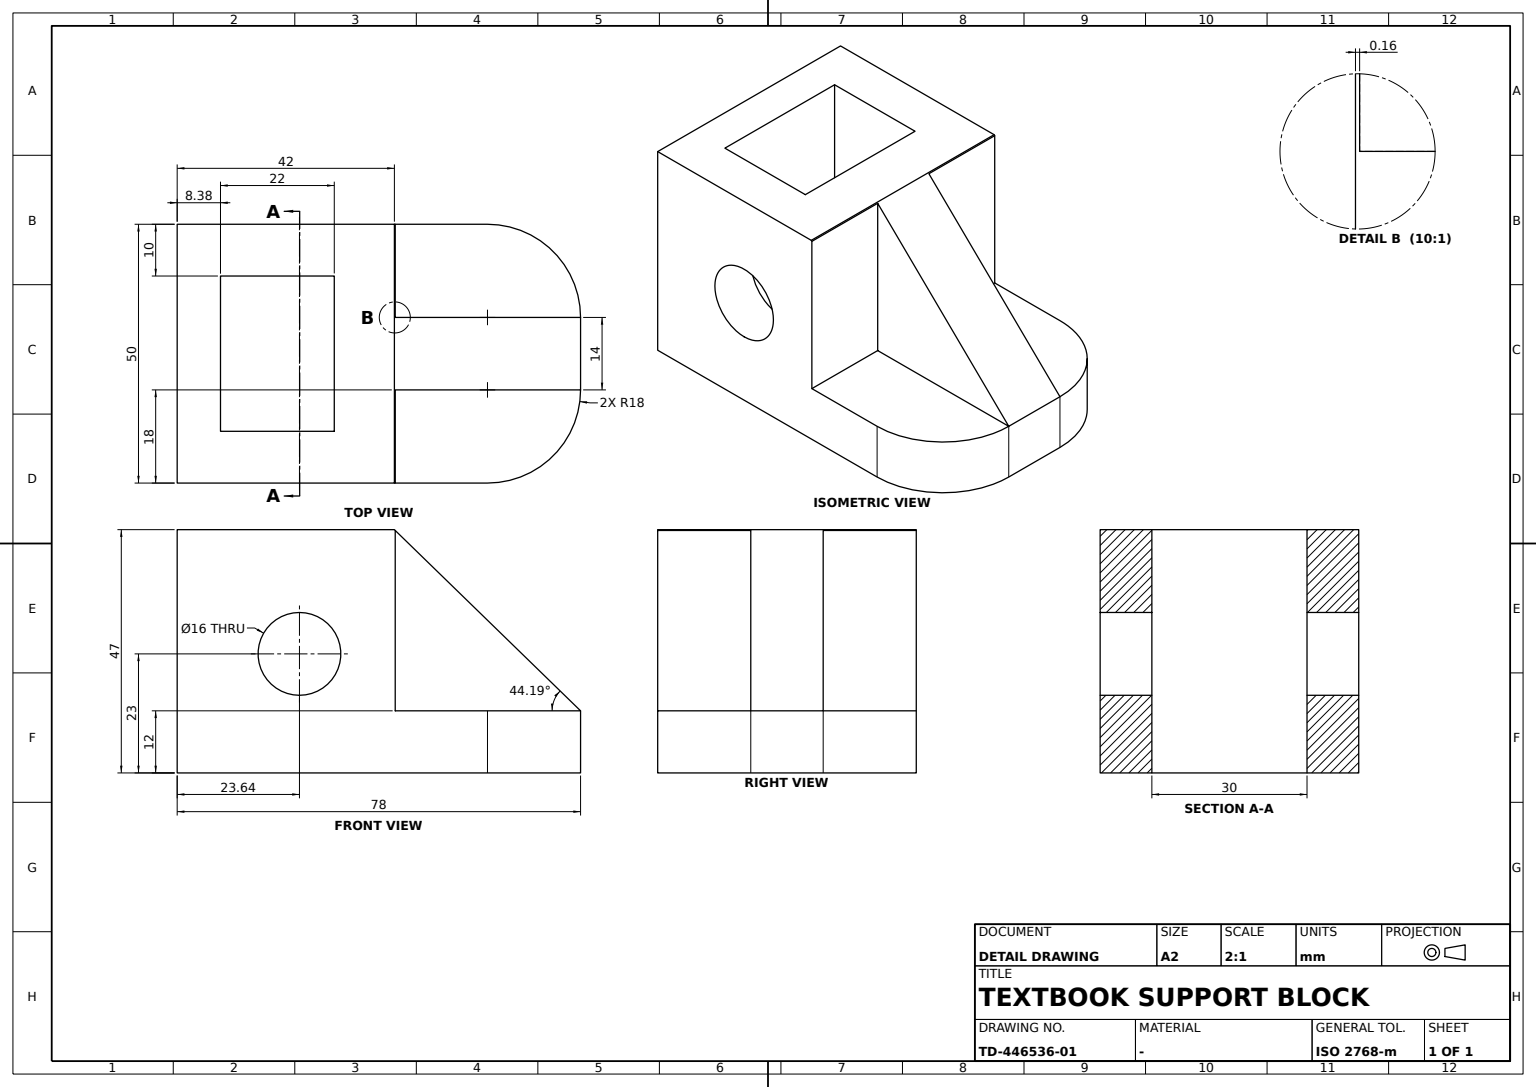
CATIA V5 part; units mm, degrees
sketch "Sketch1" plane through (0, 0, 0) normal (1, 0, 0) x (0, 1, 0)
  line L0 (0, 0) -> (0, 47)
  line L1 (0, 47) -> (78, 47)
  line L2 (78, 47) -> (78, 0)
  point P0 (78, 0)
  line L3 (78, 0) -> (0, 0)
  dimension "length L0" = 47
  dimension "length L3" = 78
  dimension "length L2" = 47
  dimension "length L1" = 78
  constraint vertical L0 y-axis
  constraint vertical L2 y-axis
  constraint horizontal L1 x-axis
  constraint horizontal L3 x-axis
  constraint coincidence P0 x-axis
extrude "Pad1" add sketch "Sketch1" along normal mid plane 50
sketch "Sketch2" plane through (25, 0, 0) normal (1, 0, 0) x (0, 1, 0)
  point P0 (42, 47)
  line L0 (42, 47) -> (78, 12)
  point P1 (78, 12)
  line L1 (78, 12) -> (78, 47)
  line L2 (78, 47) -> (42, 47)
  line L3 (0, 0) -> (78, 0) construction
  line L4 (0, 47) -> (0, 0) construction
  dimension "distance P1 L3" = 12
  dimension "distance P0 L4" = 42
  constraint vertical L1 y-axis
  constraint horizontal L2 x-axis
extrude "Pocket1" cut sketch "Sketch2" against normal through all
sketch "Sketch3" plane through (25, 0, 0) normal (1, 0, 0) x (0, 1, 0)
  point P0 (42.1607, 47)
  line L0 (42.1607, 47) -> (42.1607, 12)
  line L1 (42.1607, 12) -> (79.5614, 12)
  line L2 (0, 0) -> (78, 0) construction
  line L3 (42.1607, 47) -> (79.5614, 12)
  dimension "distance P0 L1" = 35
  dimension "distance L2 L1" = 12
  constraint vertical L0 y-axis
  constraint horizontal L1 x-axis
extrude "Pocket2" cut sketch "Sketch3" against normal blind 18
mirror "Mirror1" about plane through (0, 0, 0) normal (1, 0, 0) of "Pocket2"
fillet "Fillet1" radius 18 2 edges at (25, 78, 6) (-25, 78, 6)
sketch "Sketch4" plane through (0, 0, 47) normal (0, 0, 1) x (0, 1, 0)
  point P0 (19.3757, 0)
  line L0 (30.3757, 15) -> (30.3757, -15)
  line L1 (30.3757, -15) -> (8.3757, -15)
  line L2 (8.3757, -15) -> (8.3757, 15)
  line L3 (8.3757, 15) -> (30.3757, 15)
  dimension "length L1" = 22
  dimension "length L2" = 30
  constraint coincidence P0 x-axis
  constraint vertical L0 y-axis
  constraint vertical L2 y-axis
  constraint horizontal L1 x-axis
  constraint horizontal L3 x-axis
  constraint equidistance L0 L2 P0
  constraint equidistance L1 L3 P0
extrude "Pocket3" cut sketch "Sketch4" against normal through all
sketch "Sketch5" plane through (-25, 23.6443, 31.9567) normal (-1, 0, 0) x (0, 1, 0)
  point P0 (0, 8.9567)
  line L0 (-23.6443, 31.9567) -> (54.3557, 31.9567) construction
  dimension "distance P0 L0" = 23
  dimension "D2" = 21
hole "Hole1" at (-25, 23.6443, 23) direction (1, 0, 0) diameter 16 end through all
properties part number "catia 7"
